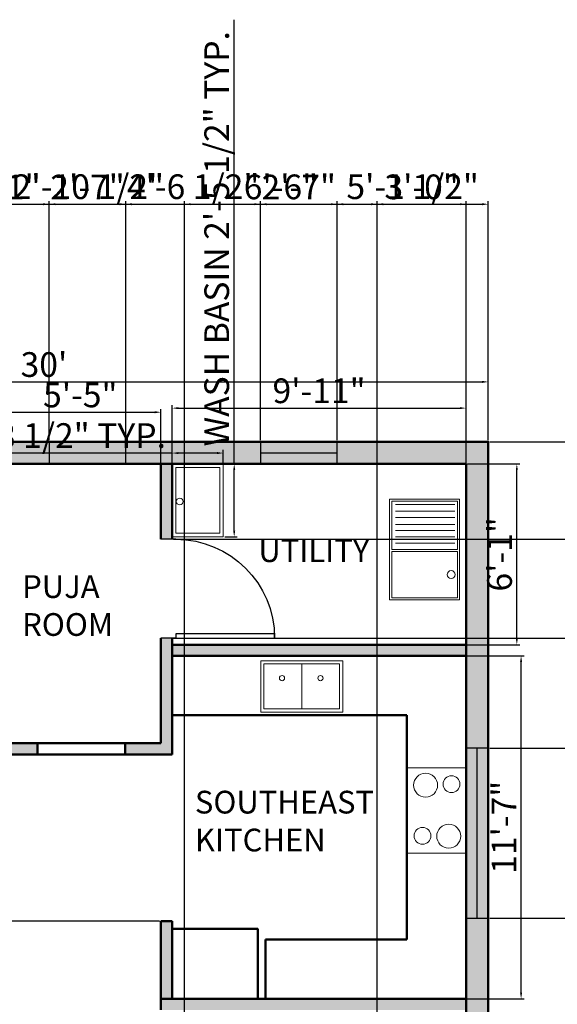
# Model space of a CAD drawing. Units: inches. Extents: x 1344 to 2521, y 3236 to 4924.
# Tile 12 of 14: x 1584 to 1801, y 4525 to 4924. Entities that reach past the tile are written whole.
import ezdxf

# ---------------------------------------------------------------- set-up
doc = ezdxf.new("R2010")
doc.units = ezdxf.units.IN
for name, color, linetype, lineweight in [('A-ANNO-DIMS', 2, 'Continuous', 18), ('A-AREA-IDEN', 3, 'Continuous', 18), ('A-DOOR', 50, 'Continuous', 25), ('A-EQPM', 9, 'Continuous', 18), ('A-FLOR-FIXT', 8, 'Continuous', 18), ('A-GLAZ', 150, 'Continuous', 25), ('A-WALL', 31, 'Continuous', 50), ('A-WALL-PATT', 8, 'Continuous', 13)]:
    doc.layers.add(name, color=color, linetype=linetype, lineweight=lineweight)
doc.styles.get("Standard").update_dxf_attribs({"font": 'arial.ttf'})
doc.dimstyles.new('ISO-25', dxfattribs={"dimtxt": 10, "dimasz": 2.5, "dimexe": 1.25, "dimexo": 0.625, "dimtad": 1, "dimdec": 0, "dimlunit": 4, "dimtxsty": 'Standard', "dimcen": 2.5, "dimadec": 0, "dimazin": 0, "dimtfac": 1, "dimtdec": 0, "dimtmove": 0, "dimatfit": 3, "dimfxl": 1, "dimarcsym": 0})

# ---------------------------------------------------------------- blocks, each defined once
blk = doc.blocks.new('*U2')
for p, q in [((0, 0), (0, -6)), ((40, 0), (40, -6))]:
    blk.add_line(p, q)
blk.add_lwpolyline([(0, 0), (0, 40), (1.75, 40), (1.75, 0)], close=True)
blk.add_arc((0, 0), 40, 0, 90)
blk = doc.blocks.new('*D15')
at = {"layer": 'A-ANNO-DIMS', "color": 0, "lineweight": -2, "transparency": 16777216}
for p, q in [((1413.52, 4753.84), (1413.52, 4778.73)), ((1416.02, 4777.48), (1771.02, 4777.48)), ((1773.52, 4753.84), (1773.52, 4778.73))]:
    blk.add_line(p, q, dxfattribs=at)
at = {"layer": 'A-ANNO-DIMS', "color": 0, "lineweight": 100, "transparency": 16777216}
for points in [[(1416.02, 4777.9), (1416.02, 4777.06), (1413.52, 4777.48)], [(1771.02, 4777.9), (1771.02, 4777.06), (1773.52, 4777.48)]]:
    blk.add_solid(points, dxfattribs=at)
at = {"layer": 'Defpoints', "color": 0, "lineweight": 100, "transparency": 16777216}
for p in [(1773.52, 4777.48), (1413.52, 4753.21), (1773.52, 4753.21)]:
    blk.add_point(p, dxfattribs=at)
at = {"layer": 'A-ANNO-DIMS', "color": 0, "transparency": 16777216, "insert": (1593.52, 4783.21), "char_height": 10, "attachment_point": 5}
blk.add_mtext("30'", dxfattribs=at)
blk = doc.blocks.new('*D19')
at = {"layer": 'A-ANNO-DIMS', "color": 0, "lineweight": -2, "transparency": 16777216}
for p, q in [((1575.52, 4744.84), (1575.52, 4766.43)), ((1578.02, 4765.18), (1638.44, 4765.18)), ((1640.94, 4744.84), (1640.94, 4766.43))]:
    blk.add_line(p, q, dxfattribs=at)
at = {"layer": 'A-ANNO-DIMS', "color": 0, "lineweight": 100, "transparency": 16777216}
for points in [[(1578.02, 4765.59), (1578.02, 4764.76), (1575.52, 4765.18)], [(1638.44, 4765.59), (1638.44, 4764.76), (1640.94, 4765.18)]]:
    blk.add_solid(points, dxfattribs=at)
at = {"layer": 'Defpoints', "color": 0, "lineweight": 100, "transparency": 16777216}
for p in [(1640.94, 4765.18), (1575.52, 4744.21), (1640.94, 4744.21)]:
    blk.add_point(p, dxfattribs=at)
at = {"layer": 'A-ANNO-DIMS', "color": 0, "transparency": 16777216, "insert": (1608.23, 4770.89), "char_height": 10, "attachment_point": 5}
blk.add_mtext('5\'-5"', dxfattribs=at)
blk = doc.blocks.new('*D20')
at = {"layer": 'A-ANNO-DIMS', "color": 0, "lineweight": -2, "transparency": 16777216}
for p, q in [((1645.44, 4744.84), (1645.44, 4768.09)), ((1764.52, 4744.84), (1764.52, 4768.09)), ((1647.94, 4766.84), (1762.02, 4766.84))]:
    blk.add_line(p, q, dxfattribs=at)
at = {"layer": 'A-ANNO-DIMS', "color": 0, "lineweight": 100, "transparency": 16777216}
for points in [[(1647.94, 4767.26), (1647.94, 4766.43), (1645.44, 4766.84)], [(1762.02, 4767.26), (1762.02, 4766.43), (1764.52, 4766.84)]]:
    blk.add_solid(points, dxfattribs=at)
at = {"layer": 'Defpoints', "color": 0, "lineweight": 100, "transparency": 16777216}
for p in [(1764.52, 4766.84), (1645.44, 4744.21), (1764.52, 4744.21)]:
    blk.add_point(p, dxfattribs=at)
at = {"layer": 'A-ANNO-DIMS', "color": 0, "transparency": 16777216, "insert": (1704.98, 4772.57), "char_height": 10, "attachment_point": 5}
blk.add_mtext('9\'-11"', dxfattribs=at)
blk = doc.blocks.new('*D30')
at = {"layer": 'A-ANNO-DIMS', "color": 0, "lineweight": -2, "transparency": 16777216}
for p, q in [((1765.14, 4666.5), (1788.07, 4666.5)), ((1786.82, 4530.04), (1786.82, 4664)), ((1765.14, 4527.54), (1788.07, 4527.54))]:
    blk.add_line(p, q, dxfattribs=at)
at = {"layer": 'A-ANNO-DIMS', "color": 0, "lineweight": 100, "transparency": 16777216}
for points in [[(1786.4, 4664), (1787.24, 4664), (1786.82, 4666.5)], [(1786.4, 4530.04), (1787.24, 4530.04), (1786.82, 4527.54)]]:
    blk.add_solid(points, dxfattribs=at)
at = {"layer": 'Defpoints', "color": 0, "lineweight": 100, "transparency": 16777216}
for p in [(1764.52, 4666.5), (1786.82, 4666.5), (1764.52, 4527.54)]:
    blk.add_point(p, dxfattribs=at)
at = {"layer": 'A-ANNO-DIMS', "color": 0, "transparency": 16777216, "insert": (1781.17, 4597.02), "char_height": 10, "attachment_point": 5, "rotation": 90}
blk.add_mtext('11\'-7"', dxfattribs=at)
blk = doc.blocks.new('*D31')
at = {"layer": 'A-ANNO-DIMS', "color": 0, "lineweight": -2, "transparency": 16777216}
for p, q in [((1765.14, 4744.21), (1786.36, 4744.21)), ((1785.11, 4673.5), (1785.11, 4741.71)), ((1765.14, 4671), (1786.36, 4671))]:
    blk.add_line(p, q, dxfattribs=at)
at = {"layer": 'A-ANNO-DIMS', "color": 0, "lineweight": 100, "transparency": 16777216}
for points in [[(1784.69, 4741.71), (1785.52, 4741.71), (1785.11, 4744.21)], [(1784.69, 4673.5), (1785.52, 4673.5), (1785.11, 4671)]]:
    blk.add_solid(points, dxfattribs=at)
at = {"layer": 'Defpoints', "color": 0, "lineweight": 100, "transparency": 16777216}
for p in [(1764.52, 4744.21), (1785.11, 4744.21), (1764.52, 4671)]:
    blk.add_point(p, dxfattribs=at)
at = {"layer": 'A-ANNO-DIMS', "color": 0, "transparency": 16777216, "insert": (1779.38, 4707.6), "char_height": 10, "attachment_point": 5, "rotation": 90}
blk.add_mtext('6\'-1"', dxfattribs=at)
blk = doc.blocks.new('WASH-BASIN')
for points in [[(29.51, 20.73), (0, 20.73), (0, 0), (29.51, 0)], [(28.05, 19.27), (1.46, 19.27), (1.46, 1.46), (28.05, 1.46)]]:
    blk.add_lwpolyline(points, close=True)
blk.add_circle((14.31, 17.66), 1.38)
blk = doc.blocks.new('*D65')
at = {"layer": 'A-ANNO-DIMS', "color": 0, "lineweight": -2, "transparency": 16777216}
for p, q in [((1670.6, 4744.21), (1670.6, 4924.22)), ((1666.8, 4744.21), (1671.85, 4744.21)), ((1670.6, 4717.2), (1670.6, 4741.71)), ((1666.8, 4714.7), (1671.85, 4714.7))]:
    blk.add_line(p, q, dxfattribs=at)
at = {"layer": 'A-ANNO-DIMS', "color": 0, "lineweight": 100, "transparency": 16777216}
for points in [[(1670.18, 4741.71), (1671.02, 4741.71), (1670.6, 4744.21)], [(1670.18, 4717.2), (1671.02, 4717.2), (1670.6, 4714.7)]]:
    blk.add_solid(points, dxfattribs=at)
at = {"layer": 'Defpoints', "color": 0, "lineweight": 100, "transparency": 16777216}
for p in [(1666.17, 4744.21), (1670.6, 4744.21), (1666.17, 4714.7)]:
    blk.add_point(p, dxfattribs=at)
at = {"layer": 'A-ANNO-DIMS', "color": 0, "transparency": 16777216, "insert": (1664.8, 4835.47), "char_height": 10, "attachment_point": 5, "rotation": 90}
blk.add_mtext('WASH BASIN 2\'-5 1/2" TYP.', dxfattribs=at)
blk = doc.blocks.new('*D66')
at = {"layer": 'A-ANNO-DIMS', "color": 0, "lineweight": -2, "transparency": 16777216}
for p, q in [((1645.44, 4748.64), (1558.38, 4748.64)), ((1645.44, 4744.84), (1645.44, 4749.89)), ((1663.67, 4748.64), (1647.94, 4748.64)), ((1666.17, 4744.84), (1666.17, 4749.89))]:
    blk.add_line(p, q, dxfattribs=at)
at = {"layer": 'A-ANNO-DIMS', "color": 0, "lineweight": 100, "transparency": 16777216}
for points in [[(1647.94, 4749.05), (1647.94, 4748.22), (1645.44, 4748.64)], [(1663.67, 4749.05), (1663.67, 4748.22), (1666.17, 4748.64)]]:
    blk.add_solid(points, dxfattribs=at)
at = {"layer": 'Defpoints', "color": 0, "lineweight": 100, "transparency": 16777216}
for p in [(1645.44, 4748.64), (1645.44, 4744.21), (1666.17, 4744.21)]:
    blk.add_point(p, dxfattribs=at)
at = {"layer": 'A-ANNO-DIMS', "color": 0, "transparency": 16777216, "insert": (1600.66, 4754.43), "char_height": 10, "attachment_point": 5}
blk.add_mtext('1\'-8 1/2" TYP.', dxfattribs=at)
blk = doc.blocks.new('*D75')
at = {"layer": 'A-ANNO-DIMS', "color": 0, "lineweight": -2, "transparency": 16777216}
for p, q in [((1558.43, 4753.84), (1558.43, 4850.71)), ((1560.93, 4849.46), (1593.16, 4849.46)), ((1595.66, 4753.84), (1595.66, 4850.71))]:
    blk.add_line(p, q, dxfattribs=at)
at = {"layer": 'A-ANNO-DIMS', "color": 0, "lineweight": 100, "transparency": 16777216}
for points in [[(1560.93, 4849.88), (1560.93, 4849.04), (1558.43, 4849.46)], [(1593.16, 4849.88), (1593.16, 4849.04), (1595.66, 4849.46)]]:
    blk.add_solid(points, dxfattribs=at)
at = {"layer": 'Defpoints', "color": 0, "lineweight": 100, "transparency": 16777216}
for p in [(1595.66, 4849.46), (1558.43, 4753.21), (1595.66, 4753.21)]:
    blk.add_point(p, dxfattribs=at)
at = {"layer": 'A-ANNO-DIMS', "color": 0, "transparency": 16777216, "insert": (1577.04, 4855.2), "char_height": 10, "attachment_point": 5}
blk.add_mtext('3\'-1"', dxfattribs=at)
blk = doc.blocks.new('*D76')
at = {"layer": 'A-ANNO-DIMS', "color": 0, "lineweight": -2, "transparency": 16777216}
for p, q in [((1595.66, 4753.84), (1595.66, 4850.71)), ((1598.16, 4849.46), (1624.19, 4849.46)), ((1626.69, 4753.84), (1626.69, 4850.71))]:
    blk.add_line(p, q, dxfattribs=at)
at = {"layer": 'A-ANNO-DIMS', "color": 0, "lineweight": 100, "transparency": 16777216}
for points in [[(1598.16, 4849.88), (1598.16, 4849.04), (1595.66, 4849.46)], [(1624.19, 4849.88), (1624.19, 4849.04), (1626.69, 4849.46)]]:
    blk.add_solid(points, dxfattribs=at)
at = {"layer": 'Defpoints', "color": 0, "lineweight": 100, "transparency": 16777216}
for p in [(1626.69, 4849.46), (1595.66, 4753.21), (1626.69, 4753.21)]:
    blk.add_point(p, dxfattribs=at)
at = {"layer": 'A-ANNO-DIMS', "color": 0, "transparency": 16777216, "insert": (1611.17, 4855.11), "char_height": 10, "attachment_point": 5}
blk.add_mtext('2\'-7"', dxfattribs=at)
blk = doc.blocks.new('*D77')
at = {"layer": 'A-ANNO-DIMS', "color": 0, "lineweight": -2, "transparency": 16777216}
for p, q in [((1626.69, 4753.84), (1626.69, 4850.71)), ((1629.19, 4849.46), (1678.73, 4849.46)), ((1681.23, 4753.84), (1681.23, 4850.71))]:
    blk.add_line(p, q, dxfattribs=at)
at = {"layer": 'A-ANNO-DIMS', "color": 0, "lineweight": 100, "transparency": 16777216}
for points in [[(1629.19, 4849.88), (1629.19, 4849.04), (1626.69, 4849.46)], [(1678.73, 4849.88), (1678.73, 4849.04), (1681.23, 4849.46)]]:
    blk.add_solid(points, dxfattribs=at)
at = {"layer": 'Defpoints', "color": 0, "lineweight": 100, "transparency": 16777216}
for p in [(1681.23, 4849.46), (1626.69, 4753.21), (1681.23, 4753.21)]:
    blk.add_point(p, dxfattribs=at)
at = {"layer": 'A-ANNO-DIMS', "color": 0, "transparency": 16777216, "insert": (1653.96, 4855.26), "char_height": 10, "attachment_point": 5}
blk.add_mtext('4\'-6 1/2"', dxfattribs=at)
blk = doc.blocks.new('*D78')
at = {"layer": 'A-ANNO-DIMS', "color": 0, "lineweight": -2, "transparency": 16777216}
for p, q in [((1681.23, 4753.84), (1681.23, 4850.71)), ((1683.73, 4849.46), (1709.76, 4849.46)), ((1712.26, 4753.84), (1712.26, 4850.71))]:
    blk.add_line(p, q, dxfattribs=at)
at = {"layer": 'A-ANNO-DIMS', "color": 0, "lineweight": 100, "transparency": 16777216}
for points in [[(1683.73, 4849.88), (1683.73, 4849.04), (1681.23, 4849.46)], [(1709.76, 4849.88), (1709.76, 4849.04), (1712.26, 4849.46)]]:
    blk.add_solid(points, dxfattribs=at)
at = {"layer": 'Defpoints', "color": 0, "lineweight": 100, "transparency": 16777216}
for p in [(1712.26, 4849.46), (1681.23, 4753.21), (1712.26, 4753.21)]:
    blk.add_point(p, dxfattribs=at)
at = {"layer": 'A-ANNO-DIMS', "color": 0, "transparency": 16777216, "insert": (1696.75, 4855.11), "char_height": 10, "attachment_point": 5}
blk.add_mtext('2\'-7"', dxfattribs=at)
blk = doc.blocks.new('*D79')
at = {"layer": 'A-ANNO-DIMS', "color": 0, "lineweight": -2, "transparency": 16777216}
for p, q in [((1712.26, 4753.84), (1712.26, 4850.71)), ((1714.76, 4849.46), (1771.02, 4849.46)), ((1773.52, 4753.84), (1773.52, 4850.71))]:
    blk.add_line(p, q, dxfattribs=at)
at = {"layer": 'A-ANNO-DIMS', "color": 0, "lineweight": 100, "transparency": 16777216}
for points in [[(1714.76, 4849.88), (1714.76, 4849.04), (1712.26, 4849.46)], [(1771.02, 4849.88), (1771.02, 4849.04), (1773.52, 4849.46)]]:
    blk.add_solid(points, dxfattribs=at)
at = {"layer": 'Defpoints', "color": 0, "lineweight": 100, "transparency": 16777216}
for p in [(1773.52, 4849.46), (1712.26, 4753.21), (1773.52, 4753.21)]:
    blk.add_point(p, dxfattribs=at)
at = {"layer": 'A-ANNO-DIMS', "color": 0, "transparency": 16777216, "insert": (1742.89, 4855.26), "char_height": 10, "attachment_point": 5}
blk.add_mtext('5\'-1 1/2"', dxfattribs=at)
blk = doc.blocks.new('*D85')
at = {"layer": 'A-ANNO-DIMS', "color": 0, "lineweight": -2, "transparency": 16777216}
for p, q in [((1774.14, 4753.21), (1820.02, 4753.21)), ((1818.77, 4750.71), (1818.77, 4631.58)), ((1774.14, 4629.08), (1820.02, 4629.08))]:
    blk.add_line(p, q, dxfattribs=at)
at = {"layer": 'A-ANNO-DIMS', "color": 0, "lineweight": 100, "transparency": 16777216}
for points in [[(1818.35, 4750.71), (1819.18, 4750.71), (1818.77, 4753.21)], [(1818.35, 4631.58), (1819.18, 4631.58), (1818.77, 4629.08)]]:
    blk.add_solid(points, dxfattribs=at)
at = {"layer": 'Defpoints', "color": 0, "lineweight": 100, "transparency": 16777216}
for p in [(1773.52, 4753.21), (1773.52, 4629.08), (1818.77, 4629.08)]:
    blk.add_point(p, dxfattribs=at)
at = {"layer": 'A-ANNO-DIMS', "color": 0, "transparency": 16777216, "insert": (1813.04, 4691.15), "char_height": 10, "attachment_point": 5, "rotation": 90}
blk.add_mtext('10\'-4"', dxfattribs=at)
blk = doc.blocks.new('*D86')
at = {"layer": 'A-ANNO-DIMS', "color": 0, "lineweight": -2, "transparency": 16777216}
for p, q in [((1774.14, 4629.08), (1820.02, 4629.08)), ((1818.77, 4626.58), (1818.77, 4562.66)), ((1774.14, 4560.16), (1820.02, 4560.16))]:
    blk.add_line(p, q, dxfattribs=at)
at = {"layer": 'A-ANNO-DIMS', "color": 0, "lineweight": 100, "transparency": 16777216}
for points in [[(1818.35, 4626.58), (1819.18, 4626.58), (1818.77, 4629.08)], [(1818.35, 4562.66), (1819.18, 4562.66), (1818.77, 4560.16)]]:
    blk.add_solid(points, dxfattribs=at)
at = {"layer": 'Defpoints', "color": 0, "lineweight": 100, "transparency": 16777216}
for p in [(1773.52, 4629.08), (1773.52, 4560.16), (1818.77, 4560.16)]:
    blk.add_point(p, dxfattribs=at)
at = {"layer": 'A-ANNO-DIMS', "color": 0, "transparency": 16777216, "insert": (1813.04, 4594.62), "char_height": 10, "attachment_point": 5, "rotation": 90}
blk.add_mtext('5\'-9"', dxfattribs=at)
blk = doc.blocks.new('*D87')
at = {"layer": 'A-ANNO-DIMS', "color": 0, "lineweight": -2, "transparency": 16777216}
for p, q in [((1774.14, 4560.16), (1820.02, 4560.16)), ((1818.77, 4557.66), (1818.77, 4496.69)), ((1774.14, 4494.19), (1820.02, 4494.19))]:
    blk.add_line(p, q, dxfattribs=at)
at = {"layer": 'A-ANNO-DIMS', "color": 0, "lineweight": 100, "transparency": 16777216}
for points in [[(1818.35, 4557.66), (1819.18, 4557.66), (1818.77, 4560.16)], [(1818.35, 4496.69), (1819.18, 4496.69), (1818.77, 4494.19)]]:
    blk.add_solid(points, dxfattribs=at)
at = {"layer": 'Defpoints', "color": 0, "lineweight": 100, "transparency": 16777216}
for p in [(1773.52, 4560.16), (1773.52, 4494.19), (1818.77, 4494.19)]:
    blk.add_point(p, dxfattribs=at)
at = {"layer": 'A-ANNO-DIMS', "color": 0, "transparency": 16777216, "insert": (1813.04, 4527.17), "char_height": 10, "attachment_point": 5, "rotation": 90}
blk.add_mtext('5\'-6"', dxfattribs=at)
blk = doc.blocks.new('*D93')
at = {"layer": 'A-ANNO-DIMS', "color": 0, "lineweight": -2, "transparency": 16777216}
for p, q in [((1526.04, 4667.09), (1526.04, 4106.71)), ((1557.42, 4667.09), (1557.42, 4106.71)), ((1528.54, 4107.96), (1554.92, 4107.96)), ((1557.42, 4107.96), (1611.23, 4107.96))]:
    blk.add_line(p, q, dxfattribs=at)
at = {"layer": 'A-ANNO-DIMS', "color": 0, "lineweight": 100, "transparency": 16777216}
for points in [[(1528.54, 4108.38), (1528.54, 4107.54), (1526.04, 4107.96)], [(1554.92, 4108.38), (1554.92, 4107.54), (1557.42, 4107.96)]]:
    blk.add_solid(points, dxfattribs=at)
at = {"layer": 'Defpoints', "color": 0, "lineweight": 100, "transparency": 16777216}
for p in [(1526.04, 4667.71), (1557.42, 4667.71), (1557.42, 4107.96)]:
    blk.add_point(p, dxfattribs=at)
at = {"layer": 'A-ANNO-DIMS', "color": 0, "transparency": 16777216, "insert": (1585.57, 4113.76), "char_height": 10, "attachment_point": 5}
blk.add_mtext('2\'-7 1/2"', dxfattribs=at)
blk = doc.blocks.new('*D94')
at = {"layer": 'A-ANNO-DIMS', "color": 0, "lineweight": -2, "transparency": 16777216}
for p, q in [((1646.07, 4713.7), (1820.02, 4713.7)), ((1818.77, 4711.2), (1818.77, 4676.2)), ((1646.07, 4673.7), (1820.02, 4673.7))]:
    blk.add_line(p, q, dxfattribs=at)
at = {"layer": 'A-ANNO-DIMS', "color": 0, "lineweight": 100, "transparency": 16777216}
for points in [[(1818.35, 4711.2), (1819.18, 4711.2), (1818.77, 4713.7)], [(1818.35, 4676.2), (1819.18, 4676.2), (1818.77, 4673.7)]]:
    blk.add_solid(points, dxfattribs=at)
at = {"layer": 'Defpoints', "color": 0, "lineweight": 100, "transparency": 16777216}
for p in [(1645.44, 4713.7), (1645.44, 4673.7), (1818.77, 4673.7)]:
    blk.add_point(p, dxfattribs=at)
at = {"layer": 'A-ANNO-DIMS', "color": 0, "transparency": 16777216, "insert": (1813.03, 4693.7), "char_height": 10, "attachment_point": 5, "rotation": 90}
blk.add_mtext('3\'-4"', dxfattribs=at)
blk = doc.blocks.new('*D96')
at = {"layer": 'A-ANNO-DIMS', "color": 0, "lineweight": -2, "transparency": 16777216}
for p, q in [((1644.82, 4626.56), (1367.02, 4626.56)), ((1368.27, 4624.06), (1368.27, 4561.53)), ((1640.32, 4559.03), (1367.02, 4559.03))]:
    blk.add_line(p, q, dxfattribs=at)
at = {"layer": 'A-ANNO-DIMS', "color": 0, "lineweight": 100, "transparency": 16777216}
for points in [[(1367.85, 4624.06), (1368.68, 4624.06), (1368.27, 4626.56)], [(1367.85, 4561.53), (1368.68, 4561.53), (1368.27, 4559.03)]]:
    blk.add_solid(points, dxfattribs=at)
at = {"layer": 'Defpoints', "color": 0, "lineweight": 100, "transparency": 16777216}
for p in [(1645.44, 4626.56), (1368.27, 4559.03), (1640.94, 4559.03)]:
    blk.add_point(p, dxfattribs=at)
at = {"layer": 'A-ANNO-DIMS', "color": 0, "transparency": 16777216, "insert": (1362.47, 4592.79), "char_height": 10, "attachment_point": 5, "rotation": 90}
blk.add_mtext('5\'-7 1/2"', dxfattribs=at)
blk = doc.blocks.new('*D99')
at = {"layer": 'A-ANNO-DIMS', "color": 0, "lineweight": -2, "transparency": 16777216}
for p, q in [((1544.94, 4337.92), (1544.94, 4850.71)), ((1547.44, 4849.46), (1577, 4849.46)), ((1579.5, 4337.92), (1579.5, 4850.71)), ((1579.5, 4849.46), (1641.07, 4849.46))]:
    blk.add_line(p, q, dxfattribs=at)
at = {"layer": 'A-ANNO-DIMS', "color": 0, "lineweight": 100, "transparency": 16777216}
for points in [[(1547.44, 4849.88), (1547.44, 4849.04), (1544.94, 4849.46)], [(1577, 4849.88), (1577, 4849.04), (1579.5, 4849.46)]]:
    blk.add_solid(points, dxfattribs=at)
at = {"layer": 'Defpoints', "color": 0, "lineweight": 100, "transparency": 16777216}
for p in [(1579.5, 4849.46), (1544.94, 4337.29), (1579.5, 4337.29)]:
    blk.add_point(p, dxfattribs=at)
at = {"layer": 'A-ANNO-DIMS', "color": 0, "transparency": 16777216, "insert": (1611.53, 4855.26), "char_height": 10, "attachment_point": 5}
blk.add_mtext('2\'-10 1/2"', dxfattribs=at)
blk = doc.blocks.new('*D101')
at = {"layer": 'A-ANNO-DIMS', "color": 0, "lineweight": -2, "transparency": 16777216}
for p, q in [((1650.52, 4387.77), (1650.52, 4850.71)), ((1653.02, 4849.46), (1726.02, 4849.46)), ((1728.52, 4387.77), (1728.52, 4850.71))]:
    blk.add_line(p, q, dxfattribs=at)
at = {"layer": 'A-ANNO-DIMS', "color": 0, "lineweight": 100, "transparency": 16777216}
for points in [[(1653.02, 4849.88), (1653.02, 4849.04), (1650.52, 4849.46)], [(1726.02, 4849.88), (1726.02, 4849.04), (1728.52, 4849.46)]]:
    blk.add_solid(points, dxfattribs=at)
at = {"layer": 'Defpoints', "color": 0, "lineweight": 100, "transparency": 16777216}
for p in [(1728.52, 4849.46), (1650.52, 4387.14), (1728.52, 4387.14)]:
    blk.add_point(p, dxfattribs=at)
at = {"layer": 'A-ANNO-DIMS', "color": 0, "transparency": 16777216, "insert": (1689.52, 4855.19), "char_height": 10, "attachment_point": 5}
blk.add_mtext('6\'-6"', dxfattribs=at)
blk = doc.blocks.new('*D102')
at = {"layer": 'A-ANNO-DIMS', "color": 0, "lineweight": -2, "transparency": 16777216}
for p, q in [((1728.52, 4387.77), (1728.52, 4850.71)), ((1731.02, 4849.46), (1762.02, 4849.46)), ((1764.52, 4387.77), (1764.52, 4850.71))]:
    blk.add_line(p, q, dxfattribs=at)
at = {"layer": 'A-ANNO-DIMS', "color": 0, "lineweight": 100, "transparency": 16777216}
for points in [[(1731.02, 4849.88), (1731.02, 4849.04), (1728.52, 4849.46)], [(1762.02, 4849.88), (1762.02, 4849.04), (1764.52, 4849.46)]]:
    blk.add_solid(points, dxfattribs=at)
at = {"layer": 'Defpoints', "color": 0, "lineweight": 100, "transparency": 16777216}
for p in [(1764.52, 4849.46), (1728.52, 4387.14), (1764.52, 4387.14)]:
    blk.add_point(p, dxfattribs=at)
at = {"layer": 'A-ANNO-DIMS', "color": 0, "transparency": 16777216, "insert": (1746.52, 4855.2), "char_height": 10, "attachment_point": 5}
blk.add_mtext('3\'-0"', dxfattribs=at)

msp = doc.modelspace()

# ---------------------------------------------------------------- hatches: boundary and pattern name
at = {"layer": 'A-WALL-PATT'}
h = msp.add_hatch(color=256, dxfattribs=at)
h.dxf.hatch_style = 1
h.paths.add_polyline_path([(1595.66, 4753.21), (1558.43, 4753.21), (1558.43, 4744.21), (1571.02, 4744.21), (1595.66, 4744.21)])
h.paths.add_polyline_path([(1681.23, 4753.21), (1626.69, 4753.21), (1626.69, 4744.21), (1681.23, 4744.21)])
h.paths.add_polyline_path([(1773.52, 4753.21), (1712.26, 4753.21), (1712.26, 4744.21), (1764.52, 4744.21), (1764.52, 4629.08), (1773.52, 4629.08)])
h.paths.add_polyline_path([(1527.4, 4753.21), (1476.83, 4753.21), (1476.83, 4744.21), (1518.52, 4744.21), (1527.4, 4744.21)])
h.paths.add_polyline_path([(1445.8, 4753.21), (1413.52, 4753.21), (1413.52, 4639.46), (1422.52, 4639.46), (1422.52, 4744.21), (1445.8, 4744.21)])
h.paths.add_polyline_path([(1523.02, 4744.21), (1518.52, 4744.21), (1518.52, 4672.21), (1515.66, 4672.21), (1515.66, 4667.71), (1523.02, 4667.71), (1526.04, 4667.71), (1526.04, 4672.21), (1523.02, 4672.21)])
h.paths.add_polyline_path([(1575.52, 4744.21), (1571.02, 4744.21), (1571.02, 4672.21), (1557.42, 4672.21), (1557.42, 4667.71), (1571.02, 4667.71), (1571.02, 4626.56), (1590.95, 4626.56), (1590.95, 4631.06), (1575.52, 4631.06), (1575.52, 4667.71)])
h.paths.add_polyline_path([(1484.28, 4672.21), (1422.52, 4672.21), (1422.52, 4667.71), (1484.28, 4667.71)])
h.paths.add_polyline_path([(1645.44, 4673.7), (1640.94, 4673.7), (1640.94, 4631.06), (1626.4, 4631.06), (1626.4, 4626.56), (1645.44, 4626.56)])
h.paths.add_polyline_path([(1645.44, 4744.21), (1640.94, 4744.21), (1640.94, 4713.7), (1645.44, 4713.7)])
h.paths.add_polyline_path([(1764.52, 4671), (1645.44, 4671), (1645.44, 4666.5), (1764.52, 4666.5)])
h.paths.add_polyline_path([(1764.52, 4527.54), (1640.94, 4527.54), (1640.94, 4523.04), (1764.52, 4523.04)])
h.paths.add_polyline_path([(1645.44, 4555.81), (1645.44, 4559.03), (1640.94, 4559.03), (1640.94, 4527.54), (1645.44, 4527.54)])
h = msp.add_hatch(color=256, dxfattribs=at)
h.dxf.hatch_style = 1
h.paths.add_polyline_path([(1773.52, 4425.27), (1764.52, 4425.27), (1764.52, 4225.22), (1743.16, 4225.22), (1743.16, 4216.22), (1764.52, 4216.22), (1764.52, 4162.21), (1764.52, 4155.88), (1653.6, 4155.88), (1653.6, 4177.58), (1764.52, 4177.58), (1764.52, 4180.4), (1649.25, 4180.4), (1649.25, 4153.21), (1773.52, 4153.21)], flags=17)
h.paths.add_polyline_path([(1598.02, 4180.38), (1593.52, 4180.38), (1589.02, 4180.38), (1589.02, 4162.21), (1565.92, 4162.21), (1565.92, 4153.21), (1598.02, 4153.21)], flags=17)
h.paths.add_polyline_path([(1689.47, 4225.22), (1666.04, 4225.22), (1666.04, 4220.75), (1666.04, 4216.22), (1689.47, 4216.22)], flags=16)
h.paths.add_polyline_path([(1442.43, 4162.21), (1422.52, 4162.21), (1422.52, 4744.21), (1764.52, 4744.21), (1764.52, 4225.22), (1743.16, 4225.22), (1743.16, 4216.22), (1764.52, 4216.22), (1764.52, 4162.21), (1764.52, 4155.88), (1653.6, 4155.88), (1653.6, 4177.58), (1764.52, 4177.58), (1764.52, 4180.4), (1649.25, 4180.4), (1649.25, 4153.21), (1773.52, 4153.21), (1773.52, 4425.27), (1773.52, 4753.21), (1413.52, 4753.21), (1413.52, 4153.21), (1442.43, 4153.21)])
h.paths.add_polyline_path([(1648.69, 4179.48), (1724.08, 4179.48), (1724.08, 4213.98), (1648.69, 4213.98)], flags=25)
h.paths.add_polyline_path([(1609.51, 4245.39), (1659.17, 4245.39), (1659.17, 4264.37), (1609.51, 4264.37)], flags=25)
h.paths.add_polyline_path([(1618.52, 4270.74), (1667.67, 4270.74), (1667.67, 4305.24), (1618.52, 4305.24)], flags=25)
h.paths.add_polyline_path([(1563.46, 4499.55), (1651.73, 4499.55), (1651.73, 4518.53), (1563.46, 4518.53)], flags=25)
h.paths.add_polyline_path([(1439.72, 4433.21), (1521.54, 4433.21), (1521.54, 4467.71), (1439.72, 4467.71)], flags=25)
h.paths.add_polyline_path([(1651.43, 4581.89), (1735.04, 4581.89), (1735.04, 4616.38), (1651.43, 4616.38)], flags=25)
h.paths.add_polyline_path([(1495.42, 4585.56), (1566.53, 4585.56), (1566.53, 4620.06), (1495.42, 4620.06)], flags=25)
h.paths.add_polyline_path([(1677.05, 4699.47), (1729.56, 4699.47), (1729.56, 4718.45), (1677.05, 4718.45)], flags=25)
h.paths.add_polyline_path([(1581.37, 4669.39), (1626.01, 4669.39), (1626.01, 4703.88), (1581.37, 4703.88)], flags=25)
h.paths.add_polyline_path([(1523.21, 4717.23), (1572.85, 4717.23), (1572.85, 4736.21), (1523.21, 4736.21)], flags=25)
h.paths.add_polyline_path([(1432.59, 4685.86), (1482.24, 4685.86), (1482.24, 4704.84), (1432.59, 4704.84)], flags=25)

# ---------------------------------------------------------------- linework, layer by layer
at = {"layer": 'A-EQPM'}
for p, q in [((1735.88, 4727.78), (1759.97, 4727.78)), ((1735.88, 4725.09), (1759.97, 4725.09)), ((1735.88, 4722.54), (1759.97, 4722.54)), ((1735.88, 4719.72), (1759.97, 4719.72)), ((1735.88, 4717.29), (1759.97, 4717.29)), ((1735.88, 4714.74), (1759.97, 4714.74)), ((1735.88, 4712.18), (1759.97, 4712.18)), ((1761.06, 4709.59), (1734.41, 4709.59)), ((1761.06, 4708.71), (1734.41, 4708.71)), ((1697.96, 4644.95), (1697.96, 4663.18))]:
    msp.add_line(p, q, dxfattribs=at)
for points in [[(1761.93, 4730.01), (1733.53, 4730.01), (1733.53, 4689.16), (1761.93, 4689.16)], [(1681.35, 4664.49), (1714.56, 4664.49), (1714.56, 4643.64), (1681.35, 4643.64)], [(1682.66, 4663.18), (1713.25, 4663.18), (1713.25, 4644.95), (1682.66, 4644.95)], [(1740.52, 4586.54), (1764.52, 4586.54), (1764.52, 4621.1), (1740.52, 4621.1)]]:
    msp.add_lwpolyline(points, close=True, dxfattribs=at)
for points in [[(1761.06, 4709.59), (1761.06, 4729.13), (1734.41, 4729.13), (1734.41, 4709.59)], [(1734.41, 4708.71), (1734.41, 4690.04), (1761.06, 4690.04), (1761.06, 4708.71)]]:
    msp.add_lwpolyline(points, dxfattribs=at)
for centre, radius in [((1758.49, 4699.41), 1.61), ((1689.98, 4657.45), 1.06), ((1705.54, 4657.45), 1.06), ((1748.14, 4614.06), 4.85), ((1758.61, 4614.48), 3.4), ((1746.86, 4593.57), 3.4), ((1757.5, 4593.39), 4.85)]:
    msp.add_circle(centre, radius, dxfattribs=at)
at = {"layer": 'A-GLAZ'}
for p, q in [((1595.66, 4748.71), (1626.69, 4748.71)), ((1681.23, 4748.71), (1712.26, 4748.71)), ((1769.02, 4560.16), (1769.02, 4629.08))]:
    msp.add_line(p, q, dxfattribs=at)
for points in [[(1595.66, 4744.21), (1626.69, 4744.21), (1626.69, 4753.21), (1595.66, 4753.21)], [(1681.23, 4744.21), (1712.26, 4744.21), (1712.26, 4753.21), (1681.23, 4753.21)], [(1764.52, 4560.16), (1773.52, 4560.16), (1773.52, 4629.08), (1764.52, 4629.08)]]:
    msp.add_lwpolyline(points, close=True, dxfattribs=at)
at = {"layer": 'A-WALL'}
for p, q in [((1640.94, 4744.21), (1640.94, 4713.7)), ((1645.44, 4744.21), (1645.44, 4713.7)), ((1640.94, 4673.7), (1640.94, 4631.06)), ((1645.44, 4673.7), (1645.44, 4626.56)), ((1645.44, 4671), (1764.52, 4671)), ((1645.44, 4666.5), (1764.52, 4666.5)), ((1645.44, 4666.5), (1645.44, 4642.5)), ((1764.52, 4666.5), (1740.52, 4666.5)), ((1645.44, 4642.5), (1740.52, 4642.5)), ((1740.52, 4642.5), (1740.52, 4551.54)), ((1590.95, 4631.06), (1575.52, 4631.06)), ((1640.94, 4631.06), (1626.4, 4631.06)), ((1590.95, 4626.56), (1571.02, 4626.56)), ((1645.44, 4626.56), (1626.4, 4626.56)), ((1640.94, 4527.54), (1640.94, 4559.03)), ((1645.44, 4559.03), (1640.94, 4559.03)), ((1645.44, 4527.54), (1645.44, 4559.03)), ((1683.24, 4527.54), (1683.24, 4551.54)), ((1683.24, 4551.54), (1740.52, 4551.54)), ((1640.94, 4527.54), (1764.52, 4527.54)), ((1640.94, 4527.54), (1640.94, 4523.04))]:
    msp.add_line(p, q, dxfattribs=at)
for points in [[(1565.92, 4153.21), (1773.52, 4153.21), (1773.52, 4753.21), (1413.52, 4753.21), (1413.52, 4153.21), (1442.43, 4153.21)], [(1764.52, 4225.22), (1764.52, 4744.21), (1422.52, 4744.21), (1422.52, 4162.21), (1442.43, 4162.21)], [(1590.95, 4626.56), (1590.95, 4631.06)], [(1626.4, 4631.06), (1626.4, 4626.56)]]:
    msp.add_lwpolyline(points, dxfattribs=at)
for points in [[(1590.95, 4626.56), (1626.4, 4626.56), (1626.4, 4631.06), (1590.95, 4631.06)], [(1645.44, 4527.54), (1680.13, 4527.54), (1680.13, 4555.81), (1645.44, 4555.81)]]:
    msp.add_lwpolyline(points, close=True, dxfattribs=at)

# ---------------------------------------------------------------- block references
at = {"layer": 'A-DOOR', "xscale": -1, "rotation": 270}
msp.add_blockref('*U2', (1646.94, 4673.7), dxfattribs=at)
at = {"layer": 'A-FLOR-FIXT', "rotation": 90.0000000000019}
msp.add_blockref('WASH-BASIN', (1666.17, 4714.71), dxfattribs=at)

# ---------------------------------------------------------------- texts
at = {"layer": 'A-AREA-IDEN', "char_height": 9.211, "attachment_point": 1}
for s, insert in [('UTILITY', (1680.36, 4713.71)), ('PUJA\\PROOM', (1584.69, 4699.14)), ('SOUTHEAST\\PKITCHEN', (1654.67, 4611.81))]:
    msp.add_mtext_dynamic_manual_height_columns(s, width=108.7809, gutter_width=46.06, heights=[0], dxfattribs=dict(at, insert=insert))

# ---------------------------------------------------------------- dimensions: what is measured, and where the dimension line sits
at = {"layer": 'A-ANNO-DIMS'}
for base, p1, p2, angle, text, picture, middle in [((1670.6, 4744.21), (1666.17, 4714.7), (1666.17, 4744.21), 90, 'WASH BASIN <> TYP.', '*D65', (1664.8, 4835.47)), ((1645.44, 4748.64), (1666.17, 4744.21), (1645.44, 4744.21), 180, '<> TYP.', '*D66', (1600.66, 4754.43))]:
    dim = msp.add_linear_dim(base=base, p1=p1, p2=p2, angle=angle, text=text, dimstyle='ISO-25', override={"dimdec": 1, "dimrnd": 0, "dimzin": 1, "dimlunit": 4, "dimfrac": 2}, dxfattribs=at)
    dim.commit()
    dim.dimension.update_dxf_attribs({"geometry": picture, "text_midpoint": middle})
for base, p1, p2, override, picture, middle in [((1579.5, 4849.46), (1544.94, 4337.29), (1579.5, 4337.29), {"dimdec": 1, "dimlfac": 1, "dimrnd": 0, "dimzin": 1, "dimdsep": 46, "dimlunit": 4, "dimfrac": 2}, '*D99', (1611.53, 4855.26)), ((1681.23, 4849.46), (1626.69, 4753.21), (1681.23, 4753.21), {"dimdec": 1, "dimlfac": 1, "dimrnd": 0, "dimzin": 1, "dimdsep": 46, "dimlunit": 4, "dimfrac": 2}, '*D77', (1653.96, 4855.26)), ((1773.52, 4849.46), (1712.26, 4753.21), (1773.52, 4753.21), {"dimdec": 1, "dimlfac": 1, "dimrnd": 0, "dimzin": 1, "dimdsep": 46, "dimlunit": 4, "dimfrac": 2}, '*D79', (1742.89, 4855.26)), ((1595.66, 4849.46), (1558.43, 4753.21), (1595.66, 4753.21), {"dimdec": 1, "dimlfac": 1, "dimrnd": 0, "dimzin": 1, "dimdsep": 46, "dimlunit": 4, "dimfrac": 2}, '*D75', (1577.04, 4855.2)), ((1626.69, 4849.46), (1595.66, 4753.21), (1626.69, 4753.21), {"dimdec": 1, "dimlfac": 1, "dimrnd": 0, "dimzin": 1, "dimdsep": 46, "dimlunit": 4, "dimfrac": 2}, '*D76', (1611.17, 4855.11)), ((1728.52, 4849.46), (1650.52, 4387.14), (1728.52, 4387.14), {"dimdec": 1, "dimlfac": 1, "dimrnd": 0, "dimzin": 1, "dimdsep": 46, "dimlunit": 4, "dimfrac": 2}, '*D101', (1689.52, 4855.19)), ((1712.26, 4849.46), (1681.23, 4753.21), (1712.26, 4753.21), {"dimdec": 1, "dimlfac": 1, "dimrnd": 0, "dimzin": 1, "dimdsep": 46, "dimlunit": 4, "dimfrac": 2}, '*D78', (1696.75, 4855.11)), ((1764.52, 4849.46), (1728.52, 4387.14), (1764.52, 4387.14), {"dimdec": 1, "dimlfac": 1, "dimrnd": 0, "dimzin": 1, "dimdsep": 46, "dimlunit": 4, "dimfrac": 2}, '*D102', (1746.52, 4855.2)), ((1773.52, 4777.48), (1413.52, 4753.21), (1773.52, 4753.21), {"dimclrd": 0, "dimclre": 0, "dimclrt": 0}, '*D15', (1593.52, 4783.21)), ((1764.52, 4766.84), (1645.44, 4744.21), (1764.52, 4744.21), {"dimclrd": 0, "dimclre": 0, "dimclrt": 0}, '*D20', (1704.98, 4772.57)), ((1640.94, 4765.18), (1575.52, 4744.21), (1640.94, 4744.21), {"dimclrd": 0, "dimclre": 0, "dimclrt": 0}, '*D19', (1608.23, 4770.89)), ((1557.42, 4107.96), (1526.04, 4667.71), (1557.42, 4667.71), {"dimdec": 1, "dimlfac": 1, "dimrnd": 0, "dimzin": 1, "dimdsep": 46, "dimlunit": 4, "dimfrac": 2}, '*D93', (1585.57, 4113.76))]:
    dim = msp.add_linear_dim(base=base, p1=p1, p2=p2, dimstyle='ISO-25', override=override, dxfattribs=at)
    dim.commit()
    dim.dimension.update_dxf_attribs({"geometry": picture, "text_midpoint": middle})
for base, p1, p2, override, picture, middle in [((1818.77, 4629.08), (1773.52, 4753.21), (1773.52, 4629.08), {"dimdec": 1, "dimlfac": 1, "dimrnd": 0, "dimzin": 1, "dimdsep": 46, "dimlunit": 4, "dimfrac": 2}, '*D85', (1813.04, 4691.15)), ((1785.11, 4744.21), (1764.52, 4671), (1764.52, 4744.21), {"dimclrd": 0, "dimclre": 0, "dimclrt": 0}, '*D31', (1779.38, 4707.6)), ((1818.77, 4673.7), (1645.44, 4713.7), (1645.44, 4673.7), {"dimdec": 1, "dimlfac": 1, "dimrnd": 0, "dimzin": 1, "dimdsep": 46, "dimlunit": 4, "dimfrac": 2}, '*D94', (1813.03, 4693.7)), ((1786.82, 4666.5), (1764.52, 4527.54), (1764.52, 4666.5), {"dimclrd": 0, "dimclre": 0, "dimclrt": 0}, '*D30', (1781.17, 4597.02)), ((1818.77, 4560.16), (1773.52, 4629.08), (1773.52, 4560.16), {"dimdec": 1, "dimlfac": 1, "dimrnd": 0, "dimzin": 1, "dimdsep": 46, "dimlunit": 4, "dimfrac": 2}, '*D86', (1813.04, 4594.62)), ((1368.27, 4559.03), (1645.44, 4626.56), (1640.94, 4559.03), {"dimdec": 1, "dimlfac": 1, "dimrnd": 0, "dimzin": 1, "dimdsep": 46, "dimlunit": 4, "dimfrac": 2}, '*D96', (1362.47, 4592.79)), ((1818.77, 4494.19), (1773.52, 4560.16), (1773.52, 4494.19), {"dimdec": 1, "dimlfac": 1, "dimrnd": 0, "dimzin": 1, "dimdsep": 46, "dimlunit": 4, "dimfrac": 2}, '*D87', (1813.04, 4527.17))]:
    dim = msp.add_linear_dim(base=base, p1=p1, p2=p2, angle=90, dimstyle='ISO-25', override=override, dxfattribs=at)
    dim.commit()
    dim.dimension.update_dxf_attribs({"geometry": picture, "text_midpoint": middle})

doc.saveas('drawing.dxf')
